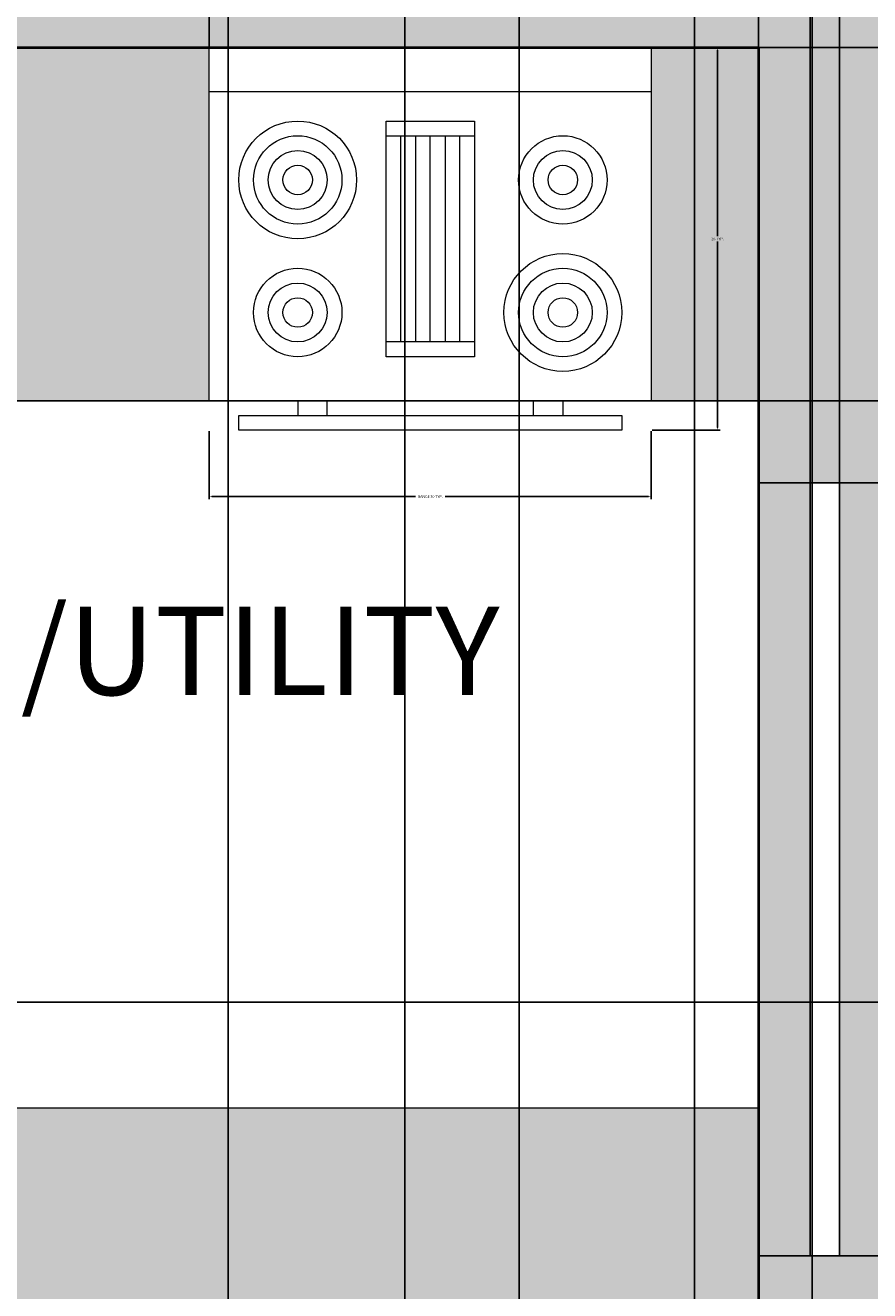
# Model space of a CAD drawing. Units: inches. Extents: x 818 to 1898, y 976 to 2364.
# Tile 90 of 96: x 1656 to 1713, y 1960 to 2046. Entities that reach past the tile are written whole.
import ezdxf

# ---------------------------------------------------------------- set-up
doc = ezdxf.new("R2010")
doc.units = ezdxf.units.IN
doc.header["$LTSCALE"] = 5
doc.header["$MEASUREMENT"] = 0
for name, color, linetype, lineweight in [('A-ANNO-DIMS', 2, 'Continuous', 18), ('A-AREA-IDEN', 7, 'Continuous', 18), ('A-EQPM', 8, 'Continuous', 18), ('A-FLOR-CASE', 8, 'Continuous', 18), ('A-FURN-PATT', 8, 'Continuous', 9), ('A-GLAZ', 4, 'Continuous', 18), ('A-WALL', 7, 'Continuous', 40)]:
    doc.layers.add(name, color=color, linetype=linetype, lineweight=lineweight)
doc.layers.add('A-GLAZ-PATT', color=141, linetype='Continuous', lineweight=9, true_color=0xadddf7)
doc.layers.add('A-WALL-PATT', color=251, linetype='Continuous', lineweight=13, true_color=0x636466)
doc.styles.get("Standard").update_dxf_attribs({"font": 'arial.ttf'})
doc.dimstyles.get("Standard").update_dxf_attribs({"dimtxt": 0.18, "dimasz": 0.18, "dimexe": 0.18, "dimexo": 0.0625, "dimgap": 0.09, "dimtad": 0, "dimtih": 1, "dimtoh": 1, "dimdec": 4, "dimzin": 0, "dimdsep": 46, "dimtxsty": 'Standard', "dimcen": 0.09, "dimadec": 0, "dimazin": 0, "dimtfac": 1, "dimtdec": 4, "dimtofl": 0, "dimtmove": 0, "dimatfit": 3, "dimfxl": 1, "dimtolj": 1, "dimtzin": 0, "dimarcsym": 0})

# ---------------------------------------------------------------- blocks, each defined once
blk = doc.blocks.new('Range-Oven - 30 in top')
for p, q in [((0, -3), (30, -3)), ((12, -6), (18, -6)), ((13, -20), (13, -6)), ((14, -6), (14, -20)), ((15, -20), (15, -6)), ((16, -6), (16, -20)), ((17, -20), (17, -6)), ((18, -20), (12, -20)), ((6, -24), (6, -25)), ((8, -25), (8, -24)), ((22, -25), (22, -24)), ((24, -24), (24, -25))]:
    blk.add_line(p, q)
for points in [[(0, -24), (0, 0), (30, 0), (30, -24)], [(12, -21), (12, -5), (18, -5), (18, -21)], [(2, -26), (2, -25), (28, -25), (28, -26)]]:
    blk.add_lwpolyline(points, close=True)
for centre, radius in [((6, -9), 4), ((6, -9), 3), ((24, -9), 3), ((6, -9), 2), ((24, -9), 2), ((6, -9), 1), ((24, -9), 1), ((24, -18), 4), ((6, -18), 3), ((24, -18), 3), ((6, -18), 2), ((24, -18), 2), ((6, -18), 1), ((24, -18), 1)]:
    blk.add_circle(centre, radius)
blk = doc.blocks.new('*D48')
at = {"layer": 'A-ANNO-DIMS', "color": 0, "lineweight": -2, "ltscale": 5, "transparency": 16777216}
for p, q in [((1668.443, 2018.016), (1668.443, 2013.398)), ((1698.443, 2018.016), (1698.443, 2013.398)), ((1668.623, 2013.578), (1682.437, 2013.578)), ((1698.263, 2013.578), (1684.448, 2013.578))]:
    blk.add_line(p, q, dxfattribs=at)
at = {"layer": 'A-ANNO-DIMS', "color": 0, "ltscale": 5, "transparency": 16777216}
for points in [[(1668.623, 2013.608), (1668.623, 2013.548), (1668.443, 2013.578)], [(1698.263, 2013.608), (1698.263, 2013.548), (1698.443, 2013.578)]]:
    blk.add_solid(points, dxfattribs=at)
at = {"layer": 'Defpoints', "color": 0, "ltscale": 5, "transparency": 16777216}
for p in [(1668.443, 2018.078), (1698.443, 2018.078), (1698.443, 2013.578)]:
    blk.add_point(p, dxfattribs=at)
at = {"layer": 'A-ANNO-DIMS', "color": 0, "ltscale": 5, "transparency": 16777216, "insert": (1683.443, 2013.578), "char_height": 0.18, "attachment_point": 5}
blk.add_mtext('\\A1;RANGE 30 TYP.', dxfattribs=at)
blk = doc.blocks.new('*D49')
at = {"layer": 'A-ANNO-DIMS', "color": 0, "lineweight": -2, "ltscale": 5, "transparency": 16777216}
for p, q in [((1698.505, 2044.078), (1703.123, 2044.078)), ((1702.943, 2043.898), (1702.943, 2031.26)), ((1702.943, 2018.258), (1702.943, 2030.896)), ((1698.505, 2018.078), (1703.123, 2018.078))]:
    blk.add_line(p, q, dxfattribs=at)
at = {"layer": 'A-ANNO-DIMS', "color": 0, "ltscale": 5, "transparency": 16777216}
for points in [[(1702.913, 2043.898), (1702.973, 2043.898), (1702.943, 2044.078)], [(1702.913, 2018.258), (1702.973, 2018.258), (1702.943, 2018.078)]]:
    blk.add_solid(points, dxfattribs=at)
at = {"layer": 'Defpoints', "color": 0, "ltscale": 5, "transparency": 16777216}
for p in [(1698.443, 2044.078), (1702.943, 2044.078), (1698.443, 2018.078)]:
    blk.add_point(p, dxfattribs=at)
at = {"layer": 'A-ANNO-DIMS', "color": 0, "ltscale": 5, "transparency": 16777216, "insert": (1702.943, 2031.078), "char_height": 0.18, "attachment_point": 5}
blk.add_mtext('\\A1;26 TYP.', dxfattribs=at)
blk = doc.blocks.new('*D85')
at = {"layer": 'A-ANNO-DIMS', "color": 0, "lineweight": -2, "ltscale": 5, "transparency": 16777216}
for p, q in [((1258.788, 2053.078), (1897.916, 2053.078)), ((1897.736, 2052.898), (1897.736, 1876.76)), ((1897.736, 1700.258), (1897.736, 1876.396)), ((1258.788, 1700.078), (1897.916, 1700.078))]:
    blk.add_line(p, q, dxfattribs=at)
at = {"layer": 'A-ANNO-DIMS', "color": 0, "ltscale": 5, "transparency": 16777216}
for points in [[(1897.706, 2052.898), (1897.766, 2052.898), (1897.736, 2053.078)], [(1897.706, 1700.258), (1897.766, 1700.258), (1897.736, 1700.078)]]:
    blk.add_solid(points, dxfattribs=at)
at = {"layer": 'Defpoints', "color": 0, "ltscale": 5, "transparency": 16777216}
for p in [(1258.725, 2053.078), (1897.736, 2053.078), (1258.725, 1700.078)]:
    blk.add_point(p, dxfattribs=at)
at = {"layer": 'A-ANNO-DIMS', "color": 0, "ltscale": 5, "transparency": 16777216, "insert": (1897.736, 1876.578), "char_height": 0.18, "attachment_point": 5}
blk.add_mtext('\\A1;353', dxfattribs=at)
blk = doc.blocks.new('*D103')
at = {"layer": 'A-ANNO-DIMS', "color": 0, "lineweight": -2, "ltscale": 5, "transparency": 16777216}
for p, q in [((1626.575, 1071.118), (1626.575, 2363.873)), ((1689.471, 1071.118), (1689.471, 2363.873)), ((1626.755, 2363.693), (1657.699, 2363.693)), ((1689.291, 2363.693), (1658.348, 2363.693))]:
    blk.add_line(p, q, dxfattribs=at)
at = {"layer": 'A-ANNO-DIMS', "color": 0, "ltscale": 5, "transparency": 16777216}
for points in [[(1626.755, 2363.723), (1626.755, 2363.663), (1626.575, 2363.693)], [(1689.291, 2363.723), (1689.291, 2363.663), (1689.471, 2363.693)]]:
    blk.add_solid(points, dxfattribs=at)
at = {"layer": 'Defpoints', "color": 0, "ltscale": 5, "transparency": 16777216}
for p in [(1689.471, 2363.693), (1626.575, 1071.055), (1689.471, 1071.055)]:
    blk.add_point(p, dxfattribs=at)
at = {"layer": 'A-ANNO-DIMS', "color": 0, "ltscale": 5, "transparency": 16777216, "insert": (1658.023, 2363.693), "char_height": 0.18, "attachment_point": 5}
blk.add_mtext('\\A1;62.9', dxfattribs=at)
blk = doc.blocks.new('*D104')
at = {"layer": 'A-ANNO-DIMS', "color": 0, "lineweight": -2, "ltscale": 5, "transparency": 16777216}
for p, q in [((1689.471, 1071.118), (1689.471, 2363.873)), ((1746.083, 1071.118), (1746.083, 2363.873)), ((1689.651, 2363.693), (1717.401, 2363.693)), ((1745.903, 2363.693), (1718.154, 2363.693))]:
    blk.add_line(p, q, dxfattribs=at)
at = {"layer": 'A-ANNO-DIMS', "color": 0, "ltscale": 5, "transparency": 16777216}
for points in [[(1689.651, 2363.723), (1689.651, 2363.663), (1689.471, 2363.693)], [(1745.903, 2363.723), (1745.903, 2363.663), (1746.083, 2363.693)]]:
    blk.add_solid(points, dxfattribs=at)
at = {"layer": 'Defpoints', "color": 0, "ltscale": 5, "transparency": 16777216}
for p in [(1746.083, 2363.693), (1689.471, 1071.055), (1746.083, 1071.055)]:
    blk.add_point(p, dxfattribs=at)
at = {"layer": 'A-ANNO-DIMS', "color": 0, "ltscale": 5, "transparency": 16777216, "insert": (1717.777, 2363.693), "char_height": 0.18, "attachment_point": 5}
blk.add_mtext('\\A1;56.61', dxfattribs=at)
blk = doc.blocks.new('*D154')
at = {"layer": 'A-ANNO-DIMS', "color": 0, "lineweight": -2, "ltscale": 5, "transparency": 16777216}
for p, q in [((1701.369, 1290.141), (1701.369, 2363.873)), ((1709.369, 1298.141), (1709.369, 2363.873)), ((1701.549, 2363.693), (1705.22, 2363.693)), ((1709.189, 2363.693), (1705.518, 2363.693))]:
    blk.add_line(p, q, dxfattribs=at)
at = {"layer": 'A-ANNO-DIMS', "color": 0, "ltscale": 5, "transparency": 16777216}
for points in [[(1701.549, 2363.723), (1701.549, 2363.663), (1701.369, 2363.693)], [(1709.189, 2363.723), (1709.189, 2363.663), (1709.369, 2363.693)]]:
    blk.add_solid(points, dxfattribs=at)
at = {"layer": 'Defpoints', "color": 0, "ltscale": 5, "transparency": 16777216}
for p in [(1709.369, 2363.693), (1709.369, 1298.078), (1701.369, 1290.078)]:
    blk.add_point(p, dxfattribs=at)
at = {"layer": 'A-ANNO-DIMS', "color": 0, "ltscale": 5, "transparency": 16777216, "insert": (1705.369, 2363.693), "char_height": 0.18, "attachment_point": 5}
blk.add_mtext('\\A1;8', dxfattribs=at)
blk = doc.blocks.new('*D175')
at = {"layer": 'A-ANNO-DIMS', "color": 0, "lineweight": -2, "ltscale": 5, "transparency": 16777216}
for p, q in [((1559.725, 1647.641), (1559.725, 2363.873)), ((1669.725, 1647.641), (1669.725, 2363.873)), ((1559.905, 2363.693), (1614.445, 2363.693)), ((1669.545, 2363.693), (1615.005, 2363.693))]:
    blk.add_line(p, q, dxfattribs=at)
at = {"layer": 'A-ANNO-DIMS', "color": 0, "ltscale": 5, "transparency": 16777216}
for points in [[(1559.905, 2363.723), (1559.905, 2363.663), (1559.725, 2363.693)], [(1669.545, 2363.723), (1669.545, 2363.663), (1669.725, 2363.693)]]:
    blk.add_solid(points, dxfattribs=at)
at = {"layer": 'Defpoints', "color": 0, "ltscale": 5, "transparency": 16777216}
for p in [(1669.725, 2363.693), (1559.725, 1647.578), (1669.725, 1647.578)]:
    blk.add_point(p, dxfattribs=at)
at = {"layer": 'A-ANNO-DIMS', "color": 0, "ltscale": 5, "transparency": 16777216, "insert": (1614.725, 2363.693), "char_height": 0.18, "attachment_point": 5}
blk.add_mtext('\\A1;110', dxfattribs=at)
blk = doc.blocks.new('*D195')
at = {"layer": 'A-ANNO-DIMS', "color": 0, "lineweight": -2, "ltscale": 5, "transparency": 16777216}
for p, q in [((1681.725, 1379.141), (1681.725, 2363.873)), ((1705.725, 1355.141), (1705.725, 2363.873)), ((1681.905, 2363.693), (1693.505, 2363.693)), ((1705.545, 2363.693), (1693.945, 2363.693))]:
    blk.add_line(p, q, dxfattribs=at)
at = {"layer": 'A-ANNO-DIMS', "color": 0, "ltscale": 5, "transparency": 16777216}
for points in [[(1681.905, 2363.723), (1681.905, 2363.663), (1681.725, 2363.693)], [(1705.545, 2363.723), (1705.545, 2363.663), (1705.725, 2363.693)]]:
    blk.add_solid(points, dxfattribs=at)
at = {"layer": 'Defpoints', "color": 0, "ltscale": 5, "transparency": 16777216}
for p in [(1705.725, 2363.693), (1681.725, 1379.078), (1705.725, 1355.078)]:
    blk.add_point(p, dxfattribs=at)
at = {"layer": 'A-ANNO-DIMS', "color": 0, "ltscale": 5, "transparency": 16777216, "insert": (1693.725, 2363.693), "char_height": 0.18, "attachment_point": 5}
blk.add_mtext('\\A1;24', dxfattribs=at)
blk = doc.blocks.new('*D203')
at = {"layer": 'A-ANNO-DIMS', "color": 0, "lineweight": -2, "ltscale": 5, "transparency": 16777216}
for p, q in [((1599.725, 1876.141), (1599.725, 2363.873)), ((1705.725, 1876.141), (1705.725, 2363.873)), ((1599.905, 2363.693), (1652.445, 2363.693)), ((1705.545, 2363.693), (1653.005, 2363.693))]:
    blk.add_line(p, q, dxfattribs=at)
at = {"layer": 'A-ANNO-DIMS', "color": 0, "ltscale": 5, "transparency": 16777216}
for points in [[(1599.905, 2363.723), (1599.905, 2363.663), (1599.725, 2363.693)], [(1705.545, 2363.723), (1705.545, 2363.663), (1705.725, 2363.693)]]:
    blk.add_solid(points, dxfattribs=at)
at = {"layer": 'Defpoints', "color": 0, "ltscale": 5, "transparency": 16777216}
for p in [(1705.725, 2363.693), (1599.725, 1876.078), (1705.725, 1876.078)]:
    blk.add_point(p, dxfattribs=at)
at = {"layer": 'A-ANNO-DIMS', "color": 0, "ltscale": 5, "transparency": 16777216, "insert": (1652.725, 2363.693), "char_height": 0.18, "attachment_point": 5}
blk.add_mtext('\\A1;106', dxfattribs=at)
blk = doc.blocks.new('*D204')
at = {"layer": 'A-ANNO-DIMS', "color": 0, "lineweight": -2, "ltscale": 5, "transparency": 16777216}
for p, q in [((1714.788, 2053.078), (1897.916, 2053.078)), ((1897.736, 2052.898), (1897.736, 1960.26)), ((1897.736, 1867.258), (1897.736, 1959.896)), ((1705.788, 1867.078), (1897.916, 1867.078))]:
    blk.add_line(p, q, dxfattribs=at)
at = {"layer": 'A-ANNO-DIMS', "color": 0, "ltscale": 5, "transparency": 16777216}
for points in [[(1897.706, 2052.898), (1897.766, 2052.898), (1897.736, 2053.078)], [(1897.706, 1867.258), (1897.766, 1867.258), (1897.736, 1867.078)]]:
    blk.add_solid(points, dxfattribs=at)
at = {"layer": 'Defpoints', "color": 0, "ltscale": 5, "transparency": 16777216}
for p in [(1714.725, 2053.078), (1897.736, 2053.078), (1705.725, 1867.078)]:
    blk.add_point(p, dxfattribs=at)
at = {"layer": 'A-ANNO-DIMS', "color": 0, "ltscale": 5, "transparency": 16777216, "insert": (1897.736, 1960.078), "char_height": 0.18, "attachment_point": 5}
blk.add_mtext('\\A1;186', dxfattribs=at)
blk = doc.blocks.new('*D205')
at = {"layer": 'A-ANNO-DIMS', "color": 0, "lineweight": -2, "ltscale": 5, "transparency": 16777216}
for p, q in [((1590.725, 2044.141), (1590.725, 2363.873)), ((1714.725, 2053.141), (1714.725, 2363.873)), ((1590.905, 2363.693), (1652.445, 2363.693)), ((1714.545, 2363.693), (1653.005, 2363.693))]:
    blk.add_line(p, q, dxfattribs=at)
at = {"layer": 'A-ANNO-DIMS', "color": 0, "ltscale": 5, "transparency": 16777216}
for points in [[(1590.905, 2363.723), (1590.905, 2363.663), (1590.725, 2363.693)], [(1714.545, 2363.723), (1714.545, 2363.663), (1714.725, 2363.693)]]:
    blk.add_solid(points, dxfattribs=at)
at = {"layer": 'Defpoints', "color": 0, "ltscale": 5, "transparency": 16777216}
for p in [(1714.725, 2363.693), (1714.725, 2053.078), (1590.725, 2044.078)]:
    blk.add_point(p, dxfattribs=at)
at = {"layer": 'A-ANNO-DIMS', "color": 0, "ltscale": 5, "transparency": 16777216, "insert": (1652.725, 2363.693), "char_height": 0.18, "attachment_point": 5}
blk.add_mtext('\\A1;124', dxfattribs=at)
blk = doc.blocks.new('*D208')
at = {"layer": 'A-ANNO-DIMS', "color": 0, "lineweight": -2, "ltscale": 5, "transparency": 16777216}
for p, q in [((1599.788, 2044.078), (1897.916, 2044.078)), ((1897.736, 2043.898), (1897.736, 2032.259)), ((1897.736, 2020.258), (1897.736, 2031.898)), ((1599.788, 2020.078), (1897.916, 2020.078))]:
    blk.add_line(p, q, dxfattribs=at)
at = {"layer": 'A-ANNO-DIMS', "color": 0, "ltscale": 5, "transparency": 16777216}
for points in [[(1897.706, 2043.898), (1897.766, 2043.898), (1897.736, 2044.078)], [(1897.706, 2020.258), (1897.766, 2020.258), (1897.736, 2020.078)]]:
    blk.add_solid(points, dxfattribs=at)
at = {"layer": 'Defpoints', "color": 0, "ltscale": 5, "transparency": 16777216}
for p in [(1599.725, 2044.078), (1897.736, 2044.078), (1599.725, 2020.078)]:
    blk.add_point(p, dxfattribs=at)
at = {"layer": 'A-ANNO-DIMS', "color": 0, "ltscale": 5, "transparency": 16777216, "insert": (1897.736, 2032.078), "char_height": 0.18, "attachment_point": 5}
blk.add_mtext('\\A1;24', dxfattribs=at)
blk = doc.blocks.new('*D209')
at = {"layer": 'A-ANNO-DIMS', "color": 0, "lineweight": -2, "ltscale": 5, "transparency": 16777216}
for p, q in [((1705.788, 2014.511), (1897.916, 2014.511)), ((1897.736, 2014.331), (1897.736, 1988.455)), ((1897.736, 1962.214), (1897.736, 1988.091)), ((1705.788, 1962.034), (1897.916, 1962.034))]:
    blk.add_line(p, q, dxfattribs=at)
at = {"layer": 'A-ANNO-DIMS', "color": 0, "ltscale": 5, "transparency": 16777216}
for points in [[(1897.706, 2014.331), (1897.766, 2014.331), (1897.736, 2014.511)], [(1897.706, 1962.214), (1897.766, 1962.214), (1897.736, 1962.034)]]:
    blk.add_solid(points, dxfattribs=at)
at = {"layer": 'Defpoints', "color": 0, "ltscale": 5, "transparency": 16777216}
for p in [(1705.725, 2014.511), (1897.736, 2014.511), (1705.725, 1962.034)]:
    blk.add_point(p, dxfattribs=at)
at = {"layer": 'A-ANNO-DIMS', "color": 0, "ltscale": 5, "transparency": 16777216, "insert": (1897.736, 1988.273), "char_height": 0.18, "attachment_point": 5}
blk.add_mtext('\\A1;52.48', dxfattribs=at)
blk = doc.blocks.new('*D213')
at = {"layer": 'A-ANNO-DIMS', "color": 0, "lineweight": -2, "ltscale": 5, "transparency": 16777216}
for p, q in [((1709.225, 1962.096), (1709.225, 2363.873)), ((1711.225, 1962.096), (1711.225, 2363.873)), ((1709.405, 2363.693), (1710.076, 2363.693)), ((1711.045, 2363.693), (1710.375, 2363.693))]:
    blk.add_line(p, q, dxfattribs=at)
at = {"layer": 'A-ANNO-DIMS', "color": 0, "ltscale": 5, "transparency": 16777216}
for points in [[(1709.405, 2363.723), (1709.405, 2363.663), (1709.225, 2363.693)], [(1711.045, 2363.723), (1711.045, 2363.663), (1711.225, 2363.693)]]:
    blk.add_solid(points, dxfattribs=at)
at = {"layer": 'Defpoints', "color": 0, "ltscale": 5, "transparency": 16777216}
for p in [(1711.225, 2363.693), (1709.225, 1962.034), (1711.225, 1962.034)]:
    blk.add_point(p, dxfattribs=at)
at = {"layer": 'A-ANNO-DIMS', "color": 0, "ltscale": 5, "transparency": 16777216, "insert": (1710.225, 2363.693), "char_height": 0.18, "attachment_point": 5}
blk.add_mtext('\\A1;2', dxfattribs=at)
blk = doc.blocks.new('*D230')
at = {"layer": 'A-ANNO-DIMS', "color": 0, "lineweight": -2, "ltscale": 5, "transparency": 16777216}
for p, q in [((1668.443, 2044.141), (1668.443, 2363.873)), ((1705.725, 2044.141), (1705.725, 2363.873)), ((1668.623, 2363.693), (1686.69, 2363.693)), ((1705.545, 2363.693), (1687.478, 2363.693))]:
    blk.add_line(p, q, dxfattribs=at)
at = {"layer": 'A-ANNO-DIMS', "color": 0, "ltscale": 5, "transparency": 16777216}
for points in [[(1668.623, 2363.723), (1668.623, 2363.663), (1668.443, 2363.693)], [(1705.545, 2363.723), (1705.545, 2363.663), (1705.725, 2363.693)]]:
    blk.add_solid(points, dxfattribs=at)
at = {"layer": 'Defpoints', "color": 0, "ltscale": 5, "transparency": 16777216}
for p in [(1705.725, 2363.693), (1668.443, 2044.078), (1705.725, 2044.078)]:
    blk.add_point(p, dxfattribs=at)
at = {"layer": 'A-ANNO-DIMS', "color": 0, "ltscale": 5, "transparency": 16777216, "insert": (1687.084, 2363.693), "char_height": 0.18, "attachment_point": 5}
blk.add_mtext('\\A1;37.28', dxfattribs=at)
blk = doc.blocks.new('*D239')
at = {"layer": 'A-ANNO-DIMS', "color": 0, "lineweight": -2, "ltscale": 5, "transparency": 16777216}
for p, q in [((1483.608, 1979.244), (1897.916, 1979.244)), ((1897.736, 1979.064), (1897.736, 1964.134)), ((1897.736, 1948.84), (1897.736, 1963.77)), ((1483.608, 1948.66), (1897.916, 1948.66))]:
    blk.add_line(p, q, dxfattribs=at)
at = {"layer": 'A-ANNO-DIMS', "color": 0, "ltscale": 5, "transparency": 16777216}
for points in [[(1897.706, 1979.064), (1897.766, 1979.064), (1897.736, 1979.244)], [(1897.706, 1948.84), (1897.766, 1948.84), (1897.736, 1948.66)]]:
    blk.add_solid(points, dxfattribs=at)
at = {"layer": 'Defpoints', "color": 0, "ltscale": 5, "transparency": 16777216}
for p in [(1483.545, 1979.244), (1897.736, 1979.244), (1483.545, 1948.66)]:
    blk.add_point(p, dxfattribs=at)
at = {"layer": 'A-ANNO-DIMS', "color": 0, "ltscale": 5, "transparency": 16777216, "insert": (1897.736, 1963.952), "char_height": 0.18, "attachment_point": 5}
blk.add_mtext('\\A1;30.584', dxfattribs=at)
blk = doc.blocks.new('*D241')
at = {"layer": 'A-ANNO-DIMS', "color": 0, "lineweight": -2, "ltscale": 5, "transparency": 16777216}
for p, q in [((1590.788, 2020.078), (1897.916, 2020.078)), ((1897.736, 2019.898), (1897.736, 1999.843)), ((1897.736, 1979.424), (1897.736, 1999.479)), ((1550.073, 1979.244), (1897.916, 1979.244))]:
    blk.add_line(p, q, dxfattribs=at)
at = {"layer": 'A-ANNO-DIMS', "color": 0, "ltscale": 5, "transparency": 16777216}
for points in [[(1897.706, 2019.898), (1897.766, 2019.898), (1897.736, 2020.078)], [(1897.706, 1979.424), (1897.766, 1979.424), (1897.736, 1979.244)]]:
    blk.add_solid(points, dxfattribs=at)
at = {"layer": 'Defpoints', "color": 0, "ltscale": 5, "transparency": 16777216}
for p in [(1590.725, 2020.078), (1897.736, 2020.078), (1550.011, 1979.244)]:
    blk.add_point(p, dxfattribs=at)
at = {"layer": 'A-ANNO-DIMS', "color": 0, "ltscale": 5, "transparency": 16777216, "insert": (1897.736, 1999.661), "char_height": 0.18, "attachment_point": 5}
blk.add_mtext('\\A1;40.83', dxfattribs=at)
blk = doc.blocks.new('*D282')
at = {"layer": 'A-ANNO-DIMS', "color": 0, "lineweight": -2, "ltscale": 5, "transparency": 16777216}
for p, q in [((1422.083, 2081.188), (1897.916, 2081.188)), ((1897.736, 2081.008), (1897.736, 1884.315)), ((1897.736, 1687.258), (1897.736, 1883.951)), ((1463.788, 1687.078), (1897.916, 1687.078))]:
    blk.add_line(p, q, dxfattribs=at)
at = {"layer": 'A-ANNO-DIMS', "color": 0, "ltscale": 5, "transparency": 16777216}
for points in [[(1897.706, 2081.008), (1897.766, 2081.008), (1897.736, 2081.188)], [(1897.706, 1687.258), (1897.766, 1687.258), (1897.736, 1687.078)]]:
    blk.add_solid(points, dxfattribs=at)
at = {"layer": 'Defpoints', "color": 0, "ltscale": 5, "transparency": 16777216}
for p in [(1422.02, 2081.188), (1897.736, 2081.188), (1463.725, 1687.078)]:
    blk.add_point(p, dxfattribs=at)
at = {"layer": 'A-ANNO-DIMS', "color": 0, "ltscale": 5, "transparency": 16777216, "insert": (1897.736, 1884.133), "char_height": 0.18, "attachment_point": 5}
blk.add_mtext('\\A1;394.1', dxfattribs=at)

msp = doc.modelspace()

# ---------------------------------------------------------------- hatches: boundary and pattern name
at = {"layer": 'A-FURN-PATT', "ltscale": 5}
h = msp.add_hatch(color=256, dxfattribs=at)
h.dxf.hatch_style = 1
h.paths.add_polyline_path([(1341.9997, 1981.5338), (1317.9034, 2001.8247), (1314.2595, 2001.8247), (1314.2595, 2004.893), (1310.1046, 2008.3917), (1303.9314, 2008.3917), (1303.9314, 1953.0408), (1308.1629, 1953.0408), (1314.2595, 1958.1746), (1314.2595, 1959.6079), (1315.9616, 1959.6079)])
h.paths.add_polyline_path([(1341.9997, 1981.5338), (1315.9616, 1959.6079), (1336.7936, 1959.6079), (1336.7936, 1953.0408), (1345.3966, 1953.0408), (1345.3966, 1959.6079), (1368.0379, 1959.6079)])
h.paths.add_polyline_path([(1402.518, 2008.3917), (1398.8475, 2008.3917), (1398.8475, 2001.8247), (1376.3134, 2001.8247), (1376.3134, 2008.3917), (1373.8948, 2008.3917), (1367.9307, 2003.3695), (1367.9307, 2001.8247), (1366.0961, 2001.8247), (1341.9997, 1981.5338), (1368.0379, 1959.6079), (1375.8366, 1953.0408), (1376.3134, 1953.0408), (1376.3134, 1959.6079), (1398.8475, 1959.6079), (1398.8475, 1953.0408), (1402.518, 1953.0408)])
h.paths.add_polyline_path([(1366.0961, 2001.8247), (1345.3966, 2001.8247), (1345.3966, 2008.3917), (1336.7936, 2008.3917), (1336.7936, 2001.8247), (1317.9034, 2001.8247), (1341.9997, 1981.5338)])
h.paths.add_polyline_path([(1336.7936, 1959.6079), (1315.9616, 1959.6079), (1314.2595, 1958.1746), (1314.2595, 1953.0408), (1336.7936, 1953.0408)], flags=17)
h.paths.add_polyline_path([(1367.9307, 1959.6079), (1345.3966, 1959.6079), (1345.3966, 1953.0408), (1367.9307, 1953.0408)], flags=17)
h.paths.add_polyline_path([(1398.8475, 1959.6079), (1376.3134, 1959.6079), (1376.3134, 1953.0408), (1398.8475, 1953.0408)], flags=17)
h.paths.add_polyline_path([(1368.0379, 1959.6079), (1367.9307, 1959.6079), (1367.9307, 1953.0408), (1375.8366, 1953.0408)], flags=17)
h.paths.add_polyline_path([(1314.2595, 1958.1746), (1308.1629, 1953.0408), (1314.2595, 1953.0408)], flags=17)
h.paths.add_polyline_path([(1315.9616, 1959.6079), (1314.2595, 1959.6079), (1314.2595, 1958.1746)], flags=16)
h.paths.add_polyline_path([(1314.2595, 2008.3917), (1310.1046, 2008.3917), (1314.2595, 2004.893)], flags=17)
h.paths.add_polyline_path([(1336.7936, 2008.3917), (1314.2595, 2008.3917), (1314.2595, 2004.893), (1317.9034, 2001.8247), (1336.7936, 2001.8247)], flags=17)
h.paths.add_polyline_path([(1314.2595, 2004.893), (1314.2595, 2001.8247), (1317.9034, 2001.8247)], flags=16)
h.paths.add_polyline_path([(1367.9307, 2008.3917), (1345.3966, 2008.3917), (1345.3966, 2001.8247), (1366.0961, 2001.8247), (1367.9307, 2003.3695)], flags=17)
h.paths.add_polyline_path([(1398.8475, 2008.3917), (1376.3134, 2008.3917), (1376.3134, 2001.8247), (1398.8475, 2001.8247)], flags=17)
h.paths.add_polyline_path([(1373.8948, 2008.3917), (1367.9307, 2008.3917), (1367.9307, 2003.3695)], flags=17)
h.paths.add_polyline_path([(1367.9307, 2003.3695), (1366.0961, 2001.8247), (1367.9307, 2001.8247)], flags=16)
h.paths.add_polyline_path([(1546.1595, 2044.0782), (1451.7698, 2044.0782), (1451.7698, 2020.0782), (1546.1595, 2020.0782)])
h.paths.add_polyline_path([(1492.0729, 2040.001, 0.431429), (1491.8238, 2040.251), (1491.3087, 2040.251, 0.415217), (1491.0729, 2040.001)], flags=16)
h.paths.add_polyline_path([(1481.8346, 2039.6036), (1511.886, 2039.6036), (1511.886, 2024.9917), (1481.8346, 2024.9917)], flags=16)
h.paths.add_polyline_path([(1491.0729, 2039.4857), (1491.0729, 2039.501), (1492.0729, 2039.501, -0.4117484), (1491.8401, 2039.251), (1491.8229, 2039.251), (1491.8229, 2039.2509, 0.4325918), (1492.0729, 2039.501), (1491.0729, 2039.501, 0.432604), (1491.3229, 2039.2509), (1491.3229, 2039.251), (1491.325, 2039.251, -0.4165823)], flags=0)
h.paths.add_polyline_path([(1485.3701, 2030.9622), (1485.3701, 2034.3556, -0.4142136), (1488.3701, 2037.3556), (1490.3421, 2037.3556, -0.0779193), (1491.0729, 2038.751), (1495.0729, 2038.751, -0.3148679), (1496.07, 2037.1201, -0.3016609), (1497.9049, 2034.3556), (1497.9049, 2030.9622, -0.4142136), (1494.9049, 2027.9622), (1488.3701, 2027.9622, -0.4142136)], flags=0)
h.paths.add_polyline_path([(1490.3229, 2035.751, 0.2655648), (1491.3229, 2036.751), (1491.3229, 2037.126), (1491.0729, 2037.126, -0.7914183), (1490.5434, 2037.251, -0.7914183), (1491.0729, 2037.376), (1491.3229, 2037.376), (1491.3229, 2037.751), (1492.0729, 2037.751), (1492.0729, 2037.376), (1492.3229, 2037.376, -0.7914183), (1492.8524, 2037.251, -0.7914183), (1492.3229, 2037.126), (1492.1491, 2037.126, -0.0866263), (1492.5376, 2036.0294, 0.1070481), (1493.0729, 2035.751), (1490.3229, 2035.751)], flags=0)
h.paths.add_polyline_path([(1491.9774, 2037.251, -1), (1491.4184, 2037.251, -1)], flags=0)
h.paths.add_polyline_path([(1500.0743, 2028.6045), (1500.0743, 2029.4074), (1510.8414, 2029.4074), (1510.8414, 2028.6045)], flags=0)
h.paths.add_polyline_path([(1500.0743, 2030.5314), (1500.0743, 2031.3342), (1510.8414, 2031.3342), (1510.8414, 2030.5314)], flags=0)
h.paths.add_polyline_path([(1500.0743, 2032.94), (1500.0743, 2033.7428), (1510.8414, 2033.7428), (1510.8414, 2032.94)], flags=0)
h.paths.add_polyline_path([(1500.0743, 2035.7499), (1500.0743, 2036.5528), (1510.8414, 2036.5528), (1510.8414, 2035.7499)], flags=0)
h.paths.add_polyline_path([(1590.7251, 2044.0782), (1576.1595, 2044.0782), (1576.1595, 2020.0782), (1590.7251, 2020.0782)])
h.paths.add_polyline_path([(1668.4429, 2044.0782), (1599.7251, 2044.0782), (1599.7251, 2020.0782), (1668.4429, 2020.0782)])
h.paths.add_polyline_path([(1621.2588, 2040.001, 0.431429), (1621.0097, 2040.251), (1620.4946, 2040.251, 0.415217), (1620.2588, 2040.001)], flags=16)
h.paths.add_polyline_path([(1611.0205, 2024.9917), (1611.0205, 2039.6036), (1641.0719, 2039.6036), (1641.0719, 2024.9917)], flags=16)
h.paths.add_polyline_path([(1620.2588, 2039.4857), (1620.2588, 2039.501), (1621.2588, 2039.501, -0.4117484), (1621.026, 2039.251), (1621.0088, 2039.251), (1621.0088, 2039.2509, 0.4325918), (1621.2588, 2039.501), (1620.2588, 2039.501, 0.432604), (1620.5088, 2039.2509), (1620.5088, 2039.251), (1620.5109, 2039.251, -0.4165823)], flags=0)
h.paths.add_polyline_path([(1614.556, 2030.9622), (1614.556, 2034.3556, -0.4142136), (1617.556, 2037.3556), (1619.528, 2037.3556, -0.0779193), (1620.2588, 2038.751), (1624.2588, 2038.751, -0.3148679), (1625.2559, 2037.1201, -0.3016609), (1627.0908, 2034.3556), (1627.0908, 2030.9622, -0.4142136), (1624.0908, 2027.9622), (1617.556, 2027.9622, -0.4142136)], flags=0)
h.paths.add_polyline_path([(1619.5088, 2035.751, 0.2655648), (1620.5088, 2036.751), (1620.5088, 2037.126), (1620.2588, 2037.126, -0.7914183), (1619.7293, 2037.251, -0.7914183), (1620.2588, 2037.376), (1620.5088, 2037.376), (1620.5088, 2037.751), (1621.2588, 2037.751), (1621.2588, 2037.376), (1621.5088, 2037.376, -0.7914183), (1622.0383, 2037.251, -0.7914183), (1621.5088, 2037.126), (1621.335, 2037.126, -0.0866263), (1621.7235, 2036.0294, 0.1070481), (1622.2588, 2035.751), (1619.5088, 2035.751)], flags=0)
h.paths.add_polyline_path([(1620.6043, 2037.251, -1), (1621.1633, 2037.251, -1)], flags=0)
h.paths.add_polyline_path([(1629.2602, 2028.6045), (1629.2602, 2029.4074), (1640.0273, 2029.4074), (1640.0273, 2028.6045)], flags=0)
h.paths.add_polyline_path([(1629.2602, 2030.5314), (1629.2602, 2031.3342), (1640.0273, 2031.3342), (1640.0273, 2030.5314)], flags=0)
h.paths.add_polyline_path([(1629.2602, 2032.94), (1629.2602, 2033.7428), (1640.0273, 2033.7428), (1640.0273, 2032.94)], flags=0)
h.paths.add_polyline_path([(1629.2602, 2035.7499), (1629.2602, 2036.5528), (1640.0273, 2036.5528), (1640.0273, 2035.7499)], flags=0)
h.paths.add_polyline_path([(1705.7251, 2044.0782), (1698.4429, 2044.0782), (1698.4429, 2020.0782), (1705.7251, 2020.0782)])
h.paths.add_polyline_path([(1705.7251, 1972.0782), (1599.7251, 1972.0782), (1599.7251, 1948.0782), (1705.7251, 1948.0782)])
h.paths.add_polyline_path([(1550.0109, 1979.2444), (1483.5451, 1979.2444), (1483.5451, 1948.6602), (1550.0109, 1948.6602)])
h.paths.add_polyline_path([(1490.2586, 1948.6602), (1488.2586, 1948.6602), (1488.2586, 1941.1742, 0.4142136), (1491.2586, 1938.1742), (1500.7446, 1938.1742, -0.4142136)])
h.paths.add_polyline_path([(1513.2306, 1941.1742), (1513.2306, 1948.6602), (1511.2306, 1948.6602, -0.4142136), (1500.7446, 1938.1742), (1510.2306, 1938.1742, 0.4142136)])
h.paths.add_polyline_path([(1518.778, 1948.6602), (1516.778, 1948.6602), (1516.778, 1941.1742, 0.4142136), (1519.778, 1938.1742), (1529.264, 1938.1742, -0.4142136)])
h.paths.add_polyline_path([(1541.75, 1941.1742), (1541.75, 1948.6602), (1539.75, 1948.6602, -0.4142136), (1529.264, 1938.1742), (1538.75, 1938.1742, 0.4142136)])
h.paths.add_polyline_path([(1590.7251, 1900.0782), (1519.6413, 1900.0782), (1519.6413, 1876.0782), (1590.7251, 1876.0782)])
at = {"layer": 'A-GLAZ-PATT', "ltscale": 5}
h = msp.add_hatch(color=256, dxfattribs=at)
h.dxf.hatch_style = 1
h.paths.add_polyline_path([(1283.8183, 1504.5782), (1206.7252, 1504.5782), (1206.7252, 1501.0782), (1283.8183, 1501.0782)])
h.paths.add_polyline_path([(1283.8183, 1510.0782), (1206.7252, 1510.0782), (1206.7252, 1506.5782), (1283.8183, 1506.5782)])
h.paths.add_polyline_path([(1490.9163, 1355.0782), (1439.7252, 1355.0782), (1439.7252, 1409.0522), (1436.2252, 1409.0522), (1436.2252, 1351.5782), (1490.9163, 1351.5782)])
h.paths.add_polyline_path([(1434.2252, 1409.0522), (1430.7252, 1409.0522), (1430.7252, 1346.0782), (1435.0799, 1346.0782), (1435.0731, 1346.1152), (1435.1501, 1346.0782), (1490.9163, 1346.0782), (1490.9163, 1349.5782), (1434.2252, 1349.5782)])
h.paths.add_polyline_path([(1714.7251, 1545.0782), (1711.2251, 1545.0782), (1711.2251, 1521.0782), (1714.7251, 1521.0782)])
h.paths.add_polyline_path([(1709.2251, 1545.0782), (1705.7251, 1545.0782), (1705.7251, 1521.0782), (1709.2251, 1521.0782)])
h.paths.add_polyline_path([(1714.7251, 1687.0782), (1711.2251, 1687.0782), (1711.2251, 1649.9029), (1714.7251, 1649.9029)])
h.paths.add_polyline_path([(1709.2251, 1687.0782), (1705.7251, 1687.0782), (1705.7251, 1649.9029), (1709.2251, 1649.9029)])
h.paths.add_polyline_path([(1709.2251, 1745.5584), (1705.7251, 1745.5584), (1705.7251, 1717.3178), (1709.2251, 1717.3178)])
h.paths.add_polyline_path([(1714.7251, 1745.5584), (1711.2251, 1745.5584), (1711.2251, 1717.3178), (1714.7251, 1717.3178)])
h.paths.add_polyline_path([(1714.7251, 2014.5114), (1711.2251, 2014.5114), (1711.2251, 1962.0338), (1714.7251, 1962.0338)])
h.paths.add_polyline_path([(1709.2251, 2014.5114), (1705.7251, 2014.5114), (1705.7251, 1962.0338), (1709.2251, 1962.0338)])
h.paths.add_polyline_path([(1538.5155, 2047.5782), (1485.1216, 2047.5782), (1485.1216, 2044.0782), (1538.5155, 2044.0782)])
h.paths.add_polyline_path([(1538.5155, 2053.0782), (1485.1216, 2053.0782), (1485.1216, 2049.5782), (1538.5155, 2049.5782)])
h.paths.add_polyline_path([(1388.0315, 2047.5782), (1330.305, 2047.5782), (1330.305, 2044.0782), (1388.0315, 2044.0782)])
h.paths.add_polyline_path([(1388.0315, 2053.0782), (1330.305, 2053.0782), (1330.305, 2049.5782), (1388.0315, 2049.5782)])
h.paths.add_polyline_path([(1262.2252, 2019.2871), (1258.7251, 2019.2871), (1258.7251, 1928.9218), (1262.2252, 1928.9218)])
h.paths.add_polyline_path([(1267.7252, 2019.2871), (1264.2252, 2019.2871), (1264.2252, 1928.9218), (1267.7252, 1928.9218)])
h.paths.add_polyline_path([(1262.2252, 1862.9652), (1258.7251, 1862.9652), (1258.7251, 1814.9652), (1262.2252, 1814.9652)])
h.paths.add_polyline_path([(1267.7252, 1862.9652), (1264.2252, 1862.9652), (1264.2252, 1814.9652), (1267.7252, 1814.9652)])
h.paths.add_polyline_path([(1262.2252, 1755.3321), (1258.7251, 1755.3321), (1258.7251, 1707.3321), (1262.2252, 1707.3321)])
h.paths.add_polyline_path([(1267.7252, 1755.3321), (1264.2252, 1755.3321), (1264.2252, 1707.3321), (1267.7252, 1707.3321)])
h.paths.add_polyline_path([(1251.9333, 1692.5782), (1206.7252, 1692.5782), (1206.7252, 1687.0782), (1251.9333, 1687.0782)])
h.paths.add_polyline_path([(1251.9333, 1700.0782), (1206.7252, 1700.0782), (1206.7252, 1694.5782), (1251.9333, 1694.5782)])
at = {"layer": 'A-WALL-PATT', "ltscale": 5}
h = msp.add_hatch(color=256, dxfattribs=at)
h.dxf.hatch_style = 1
h.paths.add_polyline_path([(1267.7252, 1928.9218), (1258.7251, 1928.9218), (1258.7251, 1913.6401), (1250.3029, 1913.6401), (1250.3029, 1878.3919), (1258.7251, 1878.3919), (1258.7251, 1862.9652), (1267.7252, 1862.9652)])
h.paths.add_polyline_path([(1267.7252, 1814.9652), (1258.7251, 1814.9652), (1258.7251, 1755.3321), (1267.7252, 1755.3321)])
h.paths.add_polyline_path([(1463.7251, 1696.0782), (1267.7252, 1696.0782), (1267.7252, 1707.3321), (1258.7251, 1707.3321), (1258.7251, 1700.0782), (1251.9333, 1700.0782), (1251.9333, 1687.0782), (1463.7251, 1687.0782)])
h.paths.add_polyline_path([(1714.7251, 1717.3178), (1705.7251, 1717.3178), (1705.7251, 1696.0782), (1599.7251, 1696.0782), (1599.7251, 1790.0782), (1705.7251, 1790.0782), (1705.7251, 1785.6125), (1714.7251, 1785.6125), (1714.7251, 1827.2125), (1705.7251, 1827.2125), (1705.7251, 1802.0782), (1599.7251, 1802.0782), (1599.7251, 1867.0782), (1705.7251, 1867.0782), (1705.7251, 1857.2125), (1714.7251, 1857.2125), (1714.7251, 1930.0316), (1741.8409, 1930.0316), (1741.8409, 1935.0316), (1714.7251, 1935.0316), (1714.7251, 1957.0338), (1741.8409, 1957.0338), (1741.8409, 1962.0338), (1714.7251, 1962.0338), (1705.7251, 1962.0338), (1705.7251, 1948.0782), (1599.7251, 1948.0782), (1599.7251, 1981.0782), (1590.7251, 1981.0782), (1590.7251, 1941.0782), (1620.7252, 1941.0782), (1705.7251, 1941.0782), (1705.7251, 1876.0782), (1599.7251, 1876.0782), (1599.7251, 1911.0782), (1590.7251, 1911.0782), (1590.7251, 1876.0782), (1429.2252, 1876.0782), (1429.2252, 1867.0782), (1511.7252, 1867.0782), (1528.593, 1867.0782), (1595.7252, 1867.0782), (1595.7252, 1773.0782), (1520.7252, 1773.0782), (1520.7252, 1837.5823), (1532.593, 1837.5823), (1532.593, 1867.0782), (1528.593, 1867.0782), (1528.593, 1841.5823), (1511.7252, 1841.5823), (1511.7252, 1744.9714), (1520.7252, 1744.9714), (1520.7252, 1761.0782), (1595.7252, 1761.0782), (1595.7252, 1696.0782), (1520.7252, 1696.0782), (1520.7252, 1716.0454), (1511.7252, 1716.0454), (1511.7252, 1696.0782), (1511.7252, 1687.0782), (1714.7251, 1687.0782)])
h.paths.add_polyline_path([(1714.7251, 2053.0782), (1714.7251, 2081.1881), (1709.7252, 2081.1881), (1709.7252, 2053.0782), (1681.6446, 2053.0782), (1681.6446, 2081.1881), (1676.6446, 2081.1881), (1676.6446, 2053.0782), (1538.5155, 2053.0782), (1538.5155, 2044.0782), (1590.7251, 2044.0782), (1590.7251, 2011.0782), (1599.7251, 2011.0782), (1599.7251, 2044.0782), (1705.7251, 2044.0782), (1705.7251, 2014.5114), (1714.7251, 2014.5114)])
h.paths.add_polyline_path([(1485.1216, 2053.0782), (1422.02, 2053.0782), (1422.02, 2081.1881), (1413.02, 2081.1881), (1413.02, 2053.0782), (1399.6356, 2053.0782), (1399.6356, 2081.1881), (1390.6356, 2081.1881), (1390.6356, 2053.0782), (1388.0315, 2053.0782), (1388.0315, 2044.0782), (1416.2743, 2044.0782), (1485.1216, 2044.0782)])
h.paths.add_polyline_path([(1330.305, 2053.0782), (1258.7251, 2053.0782), (1258.7251, 2019.2871), (1267.7252, 2019.2871), (1267.7252, 2044.0782), (1330.305, 2044.0782)])
h.paths.add_polyline_path([(1258.7251, 2053.0782), (1214.6577, 2053.0782), (1214.6577, 2044.0782), (1258.7251, 2044.0782)])
h.paths.add_polyline_path([(1214.6577, 2053.0782), (1180.349, 2053.0782), (1180.349, 2044.0782), (1214.6577, 2044.0782)])
h.paths.add_polyline_path([(1714.7251, 1639.5782), (1741.8409, 1639.5782), (1741.8409, 1643.5782), (1714.7251, 1643.5782), (1714.7251, 1649.9029), (1705.7251, 1649.9029), (1705.7251, 1600.0782), (1477.7252, 1600.0782), (1477.7252, 1591.0782), (1520.7252, 1591.0782), (1616.7252, 1591.0782), (1616.7252, 1416.6857), (1622.7252, 1416.6857), (1622.7252, 1463.0782), (1624.7252, 1463.0782), (1624.7252, 1467.0782), (1622.7252, 1467.0782), (1622.7252, 1591.0782), (1705.7251, 1591.0782), (1705.7251, 1545.0782), (1714.7251, 1545.0782), (1741.8409, 1545.0782), (1741.8409, 1549.0782), (1714.7251, 1549.0782), (1714.7251, 1593.9175), (1737.8409, 1593.9175), (1737.8409, 1597.9175), (1714.7251, 1597.9175)])
h.paths.add_polyline_path([(1674.9024, 2060.7419), (1714.7045, 2060.7419), (1714.7045, 2073.1061), (1674.9024, 2073.1061)], flags=25)
h.paths.add_polyline_path([(1394.5468, 2061.6618), (1422.2344, 2061.6618), (1422.2344, 2074.0261), (1394.5468, 2074.0261)], flags=24)

# ---------------------------------------------------------------- linework, layer by layer
at = {"layer": 'A-FLOR-CASE'}
for p, q in [((1599.7251, 2020.0782), (1705.7251, 2020.0782)), ((1599.7251, 1972.0782), (1705.7251, 1972.0782))]:
    msp.add_line(p, q, dxfattribs=at)
at = {"layer": 'A-GLAZ'}
for p, q in [((1705.7251, 2014.5114), (1714.7251, 2014.5114)), ((1709.2251, 2014.5114), (1709.2251, 1962.0338)), ((1711.2251, 2014.5114), (1711.2251, 1962.0338)), ((1705.7251, 1962.0338), (1714.7251, 1962.0338))]:
    msp.add_line(p, q, dxfattribs=at)
at = {"layer": 'A-WALL'}
for p, q in [((1599.7251, 2044.0782), (1705.7251, 2044.0782)), ((1705.7251, 2044.0782), (1705.7251, 1948.0782))]:
    msp.add_line(p, q, dxfattribs=at)

# ---------------------------------------------------------------- block references
at = {"layer": 'A-EQPM'}
msp.add_blockref('Range-Oven - 30 in top', (1668.4429, 2044.0782), dxfattribs=at)

# ---------------------------------------------------------------- texts
at = {"layer": 'A-AREA-IDEN', "ltscale": 5, "insert": (1602.387, 2006.1043), "char_height": 6, "attachment_point": 1}
msp.add_mtext_dynamic_manual_height_columns('WET KITCHEN/UTILITY\\P8\'-10" X 8\'-0"', width=118.992422, gutter_width=1, heights=[0], dxfattribs=at)

# ---------------------------------------------------------------- dimensions: what is measured, and where the dimension line sits
at = {"layer": 'A-ANNO-DIMS', "ltscale": 5}
for base, p1, p2, override, picture, middle in [((1669.7251, 2363.6929), (1559.7251, 1647.5782), (1669.7251, 1647.5782), {"dimdec": 0, "dimlfac": 1, "dimrnd": 0, "dimzin": 0, "dimdsep": 46, "dimlunit": 2}, '*D175', (1614.7251, 2363.6929)), ((1714.7251, 2363.6929), (1590.7251, 2044.0782), (1714.7251, 2053.0782), {"dimdec": 0, "dimlfac": 1, "dimrnd": 0, "dimzin": 0, "dimdsep": 46, "dimlunit": 2}, '*D205', (1652.7251, 2363.6929)), ((1705.7251, 2363.6929), (1599.7251, 1876.0782), (1705.7251, 1876.0782), {"dimdec": 0, "dimlfac": 1, "dimrnd": 0, "dimzin": 0, "dimdsep": 46, "dimlunit": 2}, '*D203', (1652.7251, 2363.6929)), ((1689.4714, 2363.6929), (1626.5748, 1071.0552), (1689.4714, 1071.0552), {"dimdec": 1, "dimlfac": 1, "dimrnd": 0, "dimzin": 0, "dimdsep": 46, "dimlunit": 2}, '*D103', (1658.0231, 2363.6929)), ((1705.7251, 2363.6929), (1668.4429, 2044.0782), (1705.7251, 2044.0782), {"dimdec": 2, "dimlfac": 1, "dimrnd": 0, "dimzin": 0, "dimdsep": 46, "dimlunit": 2}, '*D230', (1687.084, 2363.6929)), ((1705.7251, 2363.6929), (1681.7251, 1379.0782), (1705.7251, 1355.0782), {"dimdec": 0, "dimlfac": 1, "dimrnd": 0, "dimzin": 0, "dimdsep": 46, "dimlunit": 2}, '*D195', (1693.7251, 2363.6929)), ((1746.0831, 2363.6929), (1689.4714, 1071.0552), (1746.0831, 1071.0552), {"dimdec": 2, "dimlfac": 1, "dimrnd": 0, "dimzin": 0, "dimdsep": 46, "dimlunit": 2}, '*D104', (1717.7772, 2363.6929)), ((1709.3688, 2363.6929), (1701.3688, 1290.0782), (1709.3688, 1298.0782), {"dimdec": 0, "dimlfac": 1, "dimrnd": 0, "dimzin": 0, "dimdsep": 46, "dimlunit": 2}, '*D154', (1705.3688, 2363.6929)), ((1711.2251, 2363.6929), (1709.2251, 1962.0338), (1711.2251, 1962.0338), {"dimdec": 0, "dimlfac": 1, "dimrnd": 0, "dimzin": 0, "dimdsep": 46, "dimlunit": 2}, '*D213', (1710.2251, 2363.6929))]:
    dim = msp.add_linear_dim(base=base, p1=p1, p2=p2, dimstyle='Standard', override=override, dxfattribs=at)
    dim.commit()
    dim.dimension.update_dxf_attribs({"geometry": picture, "text_midpoint": middle})
for base, p1, p2, override, picture, middle in [((1897.736, 2081.1881), (1463.7251, 1687.0782), (1422.02, 2081.1881), {"dimdec": 1, "dimlfac": 1, "dimrnd": 0, "dimzin": 0, "dimdsep": 46, "dimlunit": 2}, '*D282', (1897.736, 1884.1332)), ((1897.736, 2053.0782), (1258.7251, 1700.0782), (1258.7251, 2053.0782), {"dimdec": 0, "dimlfac": 1, "dimrnd": 0, "dimzin": 0, "dimdsep": 46, "dimlunit": 2}, '*D85', (1897.736, 1876.5782)), ((1897.736, 2053.0782), (1705.7251, 1867.0782), (1714.7251, 2053.0782), {"dimdec": 0, "dimlfac": 1, "dimrnd": 0, "dimzin": 0, "dimdsep": 46, "dimlunit": 2}, '*D204', (1897.736, 1960.0782)), ((1897.736, 2044.0782), (1599.7251, 2020.0782), (1599.7251, 2044.0782), {"dimdec": 0, "dimlfac": 1, "dimrnd": 0, "dimzin": 0, "dimdsep": 46, "dimlunit": 2}, '*D208', (1897.736, 2032.0782)), ((1897.736, 2020.0782), (1550.0109, 1979.2444), (1590.7251, 2020.0782), {"dimdec": 2, "dimlfac": 1, "dimrnd": 0, "dimzin": 0, "dimdsep": 46, "dimlunit": 2}, '*D241', (1897.736, 1999.6613)), ((1897.736, 2014.5114), (1705.7251, 1962.0338), (1705.7251, 2014.5114), {"dimdec": 2, "dimlfac": 1, "dimrnd": 0, "dimzin": 0, "dimdsep": 46, "dimlunit": 2}, '*D209', (1897.736, 1988.2726)), ((1897.736, 1979.2444), (1483.5451, 1948.6602), (1483.5451, 1979.2444), {"dimdec": 3, "dimlfac": 1, "dimrnd": 0, "dimzin": 0, "dimdsep": 46, "dimlunit": 2}, '*D239', (1897.736, 1963.9523))]:
    dim = msp.add_linear_dim(base=base, p1=p1, p2=p2, angle=90, dimstyle='Standard', override=override, dxfattribs=at)
    dim.commit()
    dim.dimension.update_dxf_attribs({"geometry": picture, "text_midpoint": middle})
dim = msp.add_linear_dim(base=(1702.9429, 2044.0782), p1=(1698.4429, 2018.0782), p2=(1698.4429, 2044.0782), angle=90, text='<> TYP.', dimstyle='Standard', override={"dimdec": 0, "dimlfac": 1, "dimrnd": 0, "dimzin": 0, "dimdsep": 46, "dimlunit": 2}, dxfattribs=at)
dim.commit()
dim.dimension.update_dxf_attribs({"geometry": '*D49', "text_midpoint": (1702.9429, 2031.0782)})
dim = msp.add_linear_dim(base=(1698.4429, 2013.5782), p1=(1668.4429, 2018.0782), p2=(1698.4429, 2018.0782), text='RANGE <> TYP.', dimstyle='Standard', override={"dimdec": 0, "dimlfac": 1, "dimrnd": 0, "dimzin": 0, "dimdsep": 46, "dimlunit": 2}, dxfattribs=at)
dim.commit()
dim.dimension.update_dxf_attribs({"geometry": '*D48', "text_midpoint": (1683.4429, 2013.5782)})

doc.saveas('drawing.dxf')
